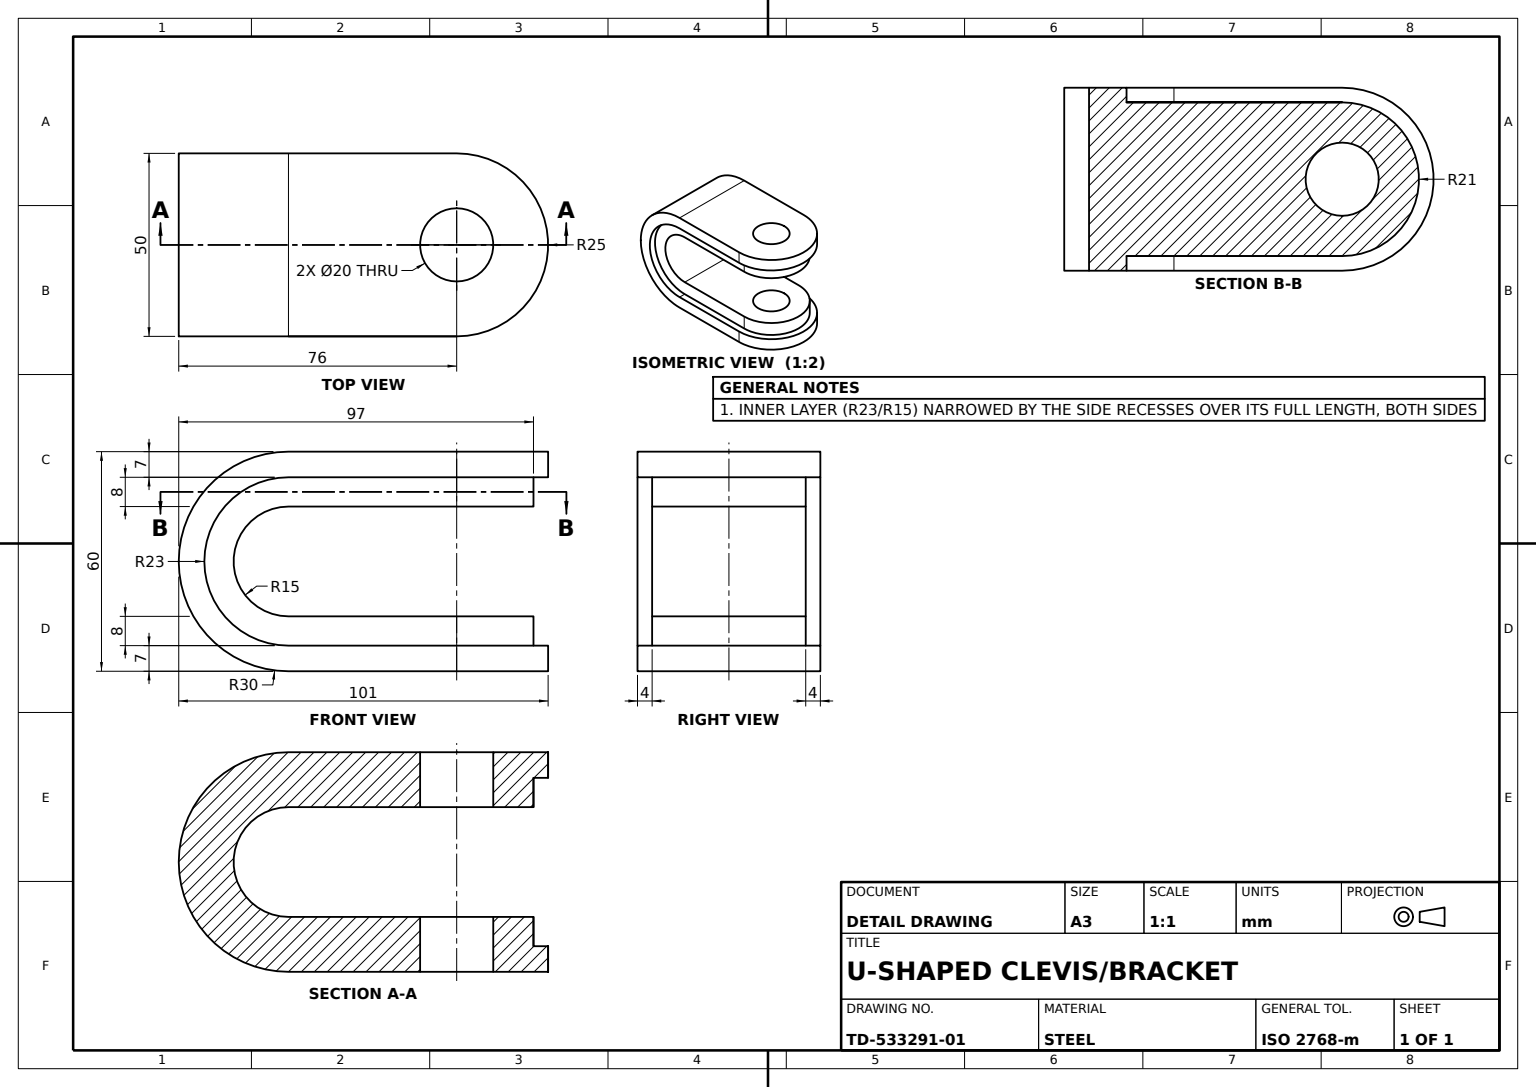
SolidWorks part; units mm, degrees
material "Plain Carbon Steel"
ref_plane "Front Plane" through (0, 0, 0) normal (0, 0, 1) x (1, 0, 0)
ref_plane "Top Plane" through (0, 0, 0) normal (0, 1, 0) x (1, 0, 0)
ref_plane "Right Plane" through (0, 0, 0) normal (1, 0, 0) x (0, 0, -1)
sketch "U Fork Profile Sketch" plane through (0, 0, 0) normal (0, 0, 1) x (1, 0, 0)
  line L1 (0, 60) -> (46, 60)
  line L3 (0, 0) -> (46, 0)
  line L4 (0, 53) -> (46, 53)
  line L5 (0, 7) -> (46, 7)
  line L6 (46, 60) -> (46, 53)
  line L7 (46, 7) -> (46, 0)
  line L8 (0, 45) -> (46, 45)
  line L10 (46, 15) -> (0, 15)
  arc A0 (0, 60) -> (0, 0) centre (0, 30) ccw
  arc A2 (0, 53) -> (0, 7) centre (0, 30) ccw
  arc A3 (0, 45) -> (0, 15) centre (0, 30) ccw
  dimension "D1" = 30
  dimension "D2" = 23
  dimension "D3" = 15
  dimension "D4" = 46
extrude "U Fork Base" add sketch "U Fork Profile Sketch" along normal blind 50 contours A2 L4 L6 L1 A0 L3 L7 L5
sketch "U Wrap Layer Sketch" plane through (0, 0, 50) normal (0, 0, 1) x (1, 0, 0)
  line L0 (0, 53) -> (46, 53)
  line L1 (0, 7) -> (46, 7)
  line L2 (0, 15) -> (46, 15)
  line L3 (46, 15) -> (46, 7)
  line L4 (0, 45) -> (46, 45)
  line L5 (46, 45) -> (46, 53)
  arc A0 (0, 45) -> (0, 15) centre (0, 30) ccw
  arc A1 (0, 53) -> (0, 7) centre (0, 30) ccw
  dimension "D1" = 15
extrude "U Wrap Layer" add sketch "U Wrap Layer Sketch" against normal blind 50
sketch "Wrap Recess 1 Sketch" plane through (0, 0, 50) normal (0, 0, 1) x (1, 0, 0)
  line L0 (0, 45) -> (46, 45)
  line L1 (0, 15) -> (46, 15)
  line L2 (46, 60) -> (46, 45) construction
  line L3 (0, 53) -> (46, 53)
  line L4 (46, 53) -> (46, 45)
  line L5 (0, 7) -> (46, 7)
  line L6 (46, 15) -> (46, 0) construction
  line L7 (46, 7) -> (46, 15)
  arc A0 (0, 45) -> (0, 15) centre (0, 30) ccw
  arc A1 (0, 53) -> (0, 7) centre (0, 30) ccw
  dimension "D1" = 23
extrude "Wrap Recess 1" cut sketch "Wrap Recess 1 Sketch" against normal blind 4
sketch "Wrap Recess 2 Sketch" plane through (0, 0, 0) normal (0, 0, -1) x (-1, 0, 0)
  line L0 (-46, 45) -> (0, 45)
  line L1 (-46, 15) -> (0, 15)
  line L2 (0, 53) -> (-46, 53)
  line L3 (-46, 60) -> (-46, 45) construction
  line L4 (-46, 53) -> (-46, 45)
  line L5 (0, 7) -> (-46, 7)
  line L6 (-46, 7) -> (-46, 15)
  arc A0 (0, 15) -> (0, 45) centre (0, 30) ccw
  arc A1 (0, 7) -> (0, 53) centre (0, 30) ccw
extrude "Wrap Recess 2" cut sketch "Wrap Recess 2 Sketch" against normal blind 4
sketch "Arm Pad 1 Sketch" plane through (0, 45, 0) normal (0, -1, 0) x (1, 0, 0)
  line L0 (46, 50) -> (46, 0) construction
  line L1 (46, 48) -> (46, 2)
  arc A0 (46, 10) -> (46, 40) centre (46, 25) ccw
  arc A1 (46, 2) -> (46, 48) centre (46, 25) ccw
  dimension "D1" = 15
  dimension "D2" = 23
extrude "Arm Pad 1" add sketch "Arm Pad 1 Sketch" against normal blind 8 contours L1 A0
sketch "Arm Pad 2 Sketch" plane through (0, 45, 0) normal (0, -1, 0) x (1, 0, 0)
  line L0 (46, 50) -> (46, 0) construction
  line L1 (46, 46) -> (46, 40)
  line L2 (46, 10) -> (46, 4)
  arc A0 (46, 10) -> (46, 40) centre (46, 25) ccw
  arc A1 (46, 4) -> (46, 46) centre (46, 25) ccw
extrude "Arm Pad 2" add sketch "Arm Pad 2 Sketch" against normal blind 8
sketch "Arm Pad 3 Sketch" plane through (0, 15, 0) normal (0, 1, 0) x (1, 0, 0)
  line L0 (46, -50) -> (46, 0) construction
  line L1 (46, -4) -> (46, -46)
  arc A0 (46, -46) -> (46, -4) centre (46, -25) ccw
  arc A1 (46, -40) -> (46, -10) centre (46, -25) ccw
  line M1 (46, -46) -> (46, -4)
  dimension "D1" = 15
extrude "Arm Pad 3" add sketch "Arm Pad 3 Sketch" against normal blind 8 contours L1 A1 | A1 A0 M1
sketch "Arm Pad 4 Sketch" plane through (0, 60, 0) normal (0, 1, 0) x (1, 0, 0)
  line L0 (46, 0) -> (46, -50)
  arc A0 (46, -50) -> (46, 0) centre (46, -25) ccw
  arc A1 (46, -46) -> (46, -4) centre (46, -25) ccw
  line M4 (46, -50) -> (46, 0)
  dimension "D1" = 25
  dimension "D2" = 21
extrude "Arm Pad 4" add sketch "Arm Pad 4 Sketch" against normal blind 8 contours A1 A0 M4 | L0 A1
sketch "Arm Pad 5 Sketch" plane through (0, 0, 0) normal (0, -1, 0) x (1, 0, 0)
  line L0 (46, 46) -> (46, 4) construction
  line L1 (46, 50) -> (46, 0)
  arc A0 (46, 0) -> (46, 50) centre (46, 25) ccw
  arc A1 (46, 4) -> (46, 46) centre (46, 25) ccw
  dimension "D1" = 21
extrude "Arm Pad 5" add sketch "Arm Pad 5 Sketch" against normal blind 8 contours L1 A1
sketch "Pin Hole Sketch" plane through (0, 0, 0) normal (0, -1, 0) x (1, 0, 0)
  circle A0 centre (46, 25) radius 10
  dimension "D1" = 20
extrude "Pin Hole" cut sketch "Pin Hole Sketch" against normal blind 70
sketch "Face Relief 1 Sketch" plane through (0, 52, 0) normal (0, -1, 0) x (1, 0, 0)
  line L0 (46, 50) -> (46, 46)
  line L1 (46, 4) -> (46, 0)
  arc A0 (46, 4) -> (46, 46) centre (46, 25) ccw
  arc A1 (46, 0) -> (46, 50) centre (46, 25) ccw
  dimension "D1" = 21
extrude "Face Relief 1" cut sketch "Face Relief 1 Sketch" against normal blind 1
sketch "Face Relief 2 Sketch" plane through (0, 8, 0) normal (0, 1, 0) x (1, 0, 0)
  line L0 (46, 0) -> (46, -4)
  line L1 (46, -46) -> (46, -50)
  arc A0 (46, -50) -> (46, 0) centre (46, -25) ccw
  arc A1 (46, -46) -> (46, -4) centre (46, -25) ccw
  dimension "D1" = 21
extrude "Face Relief 2" cut sketch "Face Relief 2 Sketch" against normal blind 1
